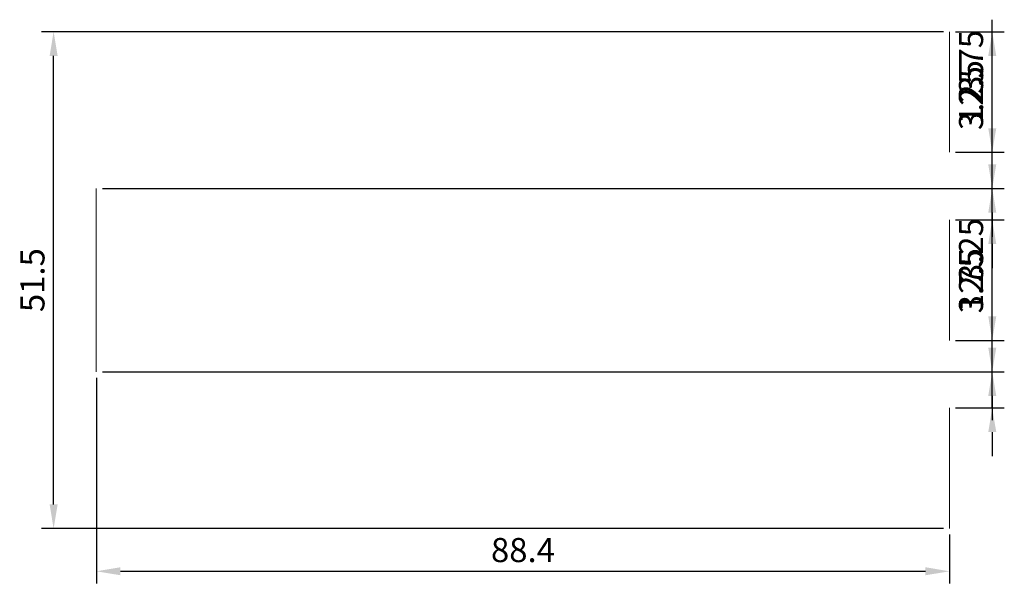
# Model space of a CAD drawing. Units: millimetres. Extents: x 330 to 432, y -31 to 27.
import ezdxf

# ---------------------------------------------------------------- set-up
doc = ezdxf.new("R2010")
doc.units = ezdxf.units.MM
doc.layers.add('M-CONS', color=8, linetype='Continuous', lineweight=13)
doc.layers.add('M-DIMS', color=2, linetype='Continuous', lineweight=18)
doc.dimstyles.new('ISO-25', dxfattribs={"dimtxt": 2.5, "dimasz": 2.5, "dimexe": 1.25, "dimexo": 0.625, "dimtad": 1, "dimtxsty": 'Standard', "dimcen": 2.5, "dimadec": 0, "dimazin": 0, "dimtfac": 1, "dimtmove": 0, "dimatfit": 3, "dimfxl": 1, "dimarcsym": 0})

# ---------------------------------------------------------------- blocks, each defined once
blk = doc.blocks.new('*D1')
at = {"layer": 'Defpoints', "color": 0, "transparency": 16777216}
for p in [(338.36, -9.5), (426.76, -25.75), (426.76, -30.18)]:
    blk.add_point(p, dxfattribs=at)
at = {"layer": 'M-DIMS', "color": 0, "lineweight": -2, "transparency": 16777216}
for p, q in [((338.36, -10.12), (338.36, -31.43)), ((426.76, -26.38), (426.76, -31.43)), ((340.86, -30.18), (424.26, -30.18))]:
    blk.add_line(p, q, dxfattribs=at)
at = {"layer": 'M-DIMS', "color": 0, "transparency": 16777216}
for points in [[(340.86, -29.76), (340.86, -30.59), (338.36, -30.18)], [(424.26, -29.76), (424.26, -30.59), (426.76, -30.18)]]:
    blk.add_solid(points, dxfattribs=at)
at = {"layer": 'M-DIMS', "color": 0, "transparency": 16777216, "insert": (382.56, -28.3), "char_height": 2.5, "attachment_point": 5}
blk.add_mtext('88.4', dxfattribs=at)
blk = doc.blocks.new('*D2')
at = {"layer": 'Defpoints', "color": 0, "transparency": 16777216}
for p in [(333.93, 25.75), (426.76, 25.75), (426.76, -25.75)]:
    blk.add_point(p, dxfattribs=at)
at = {"layer": 'M-DIMS', "color": 0, "lineweight": -2, "transparency": 16777216}
for p, q in [((426.13, 25.75), (332.68, 25.75)), ((333.93, -23.25), (333.93, 23.25)), ((426.13, -25.75), (332.68, -25.75))]:
    blk.add_line(p, q, dxfattribs=at)
at = {"layer": 'M-DIMS', "color": 0, "transparency": 16777216}
for points in [[(333.52, 23.25), (334.35, 23.25), (333.93, 25.75)], [(333.52, -23.25), (334.35, -23.25), (333.93, -25.75)]]:
    blk.add_solid(points, dxfattribs=at)
at = {"layer": 'M-DIMS', "color": 0, "transparency": 16777216, "insert": (332.06, 0), "char_height": 2.5, "attachment_point": 5, "rotation": 90}
blk.add_mtext('51.5', dxfattribs=at)
blk = doc.blocks.new('*D3')
at = {"layer": 'Defpoints', "color": 0, "transparency": 16777216}
for p in [(426.76, 25.75), (431.18, 25.75), (426.76, 13.25)]:
    blk.add_point(p, dxfattribs=at)
at = {"layer": 'M-DIMS', "color": 0, "lineweight": -2, "transparency": 16777216}
for p, q in [((427.38, 25.75), (432.43, 25.75)), ((431.18, 15.75), (431.18, 23.25)), ((427.38, 13.25), (432.43, 13.25))]:
    blk.add_line(p, q, dxfattribs=at)
at = {"layer": 'M-DIMS', "color": 0, "transparency": 16777216}
for points in [[(430.77, 23.25), (431.6, 23.25), (431.18, 25.75)], [(430.77, 15.75), (431.6, 15.75), (431.18, 13.25)]]:
    blk.add_solid(points, dxfattribs=at)
at = {"layer": 'M-DIMS', "color": 0, "transparency": 16777216, "insert": (429.31, 19.5), "char_height": 2.5, "attachment_point": 5, "rotation": 90}
blk.add_mtext('12.5', dxfattribs=at)
blk = doc.blocks.new('*D4')
at = {"layer": 'Defpoints', "color": 0, "transparency": 16777216}
for p in [(426.76, 13.25), (431.18, 13.25), (338.36, 9.5)]:
    blk.add_point(p, dxfattribs=at)
at = {"layer": 'M-DIMS', "color": 0, "lineweight": -2, "transparency": 16777216}
for p, q in [((431.18, 15.75), (431.18, 27)), ((427.38, 13.25), (432.43, 13.25)), ((431.18, 9.5), (431.18, 13.25)), ((338.98, 9.5), (432.43, 9.5)), ((431.18, 7), (431.18, 4.5))]:
    blk.add_line(p, q, dxfattribs=at)
at = {"layer": 'M-DIMS', "color": 0, "transparency": 16777216}
for points in [[(430.77, 15.75), (431.6, 15.75), (431.18, 13.25)], [(430.77, 7), (431.6, 7), (431.18, 9.5)]]:
    blk.add_solid(points, dxfattribs=at)
at = {"layer": 'M-DIMS', "color": 0, "transparency": 16777216, "insert": (429.31, 22.62), "char_height": 2.5, "attachment_point": 5, "rotation": 90}
blk.add_mtext('3.75', dxfattribs=at)
blk = doc.blocks.new('*D5')
at = {"layer": 'Defpoints', "color": 0, "transparency": 16777216}
for p in [(338.36, 9.5), (431.18, 9.5), (426.76, 6.25)]:
    blk.add_point(p, dxfattribs=at)
at = {"layer": 'M-DIMS', "color": 0, "lineweight": -2, "transparency": 16777216}
for p, q in [((431.18, 12), (431.18, 23.25)), ((338.98, 9.5), (432.43, 9.5)), ((431.18, 6.25), (431.18, 9.5)), ((427.38, 6.25), (432.43, 6.25)), ((431.18, 3.75), (431.18, 1.25))]:
    blk.add_line(p, q, dxfattribs=at)
at = {"layer": 'M-DIMS', "color": 0, "transparency": 16777216}
for points in [[(430.77, 12), (431.6, 12), (431.18, 9.5)], [(430.77, 3.75), (431.6, 3.75), (431.18, 6.25)]]:
    blk.add_solid(points, dxfattribs=at)
at = {"layer": 'M-DIMS', "color": 0, "transparency": 16777216, "insert": (429.31, 18.87), "char_height": 2.5, "attachment_point": 5, "rotation": 90}
blk.add_mtext('3.25', dxfattribs=at)
blk = doc.blocks.new('*D6')
at = {"layer": 'Defpoints', "color": 0, "transparency": 16777216}
for p in [(426.76, 6.25), (431.18, 6.25), (426.76, -6.25)]:
    blk.add_point(p, dxfattribs=at)
at = {"layer": 'M-DIMS', "color": 0, "lineweight": -2, "transparency": 16777216}
for p, q in [((427.38, 6.25), (432.43, 6.25)), ((431.18, -3.75), (431.18, 3.75)), ((427.38, -6.25), (432.43, -6.25))]:
    blk.add_line(p, q, dxfattribs=at)
at = {"layer": 'M-DIMS', "color": 0, "transparency": 16777216}
for points in [[(430.77, 3.75), (431.6, 3.75), (431.18, 6.25)], [(430.77, -3.75), (431.6, -3.75), (431.18, -6.25)]]:
    blk.add_solid(points, dxfattribs=at)
at = {"layer": 'M-DIMS', "color": 0, "transparency": 16777216, "insert": (429.31, 0), "char_height": 2.5, "attachment_point": 5, "rotation": 90}
blk.add_mtext('12.5', dxfattribs=at)
blk = doc.blocks.new('*D7')
at = {"layer": 'Defpoints', "color": 0, "transparency": 16777216}
for p in [(426.76, -6.25), (431.18, -6.25), (338.36, -9.5)]:
    blk.add_point(p, dxfattribs=at)
at = {"layer": 'M-DIMS', "color": 0, "lineweight": -2, "transparency": 16777216}
for p, q in [((431.18, -3.75), (431.18, 7.5)), ((427.38, -6.25), (432.43, -6.25)), ((431.18, -9.5), (431.18, -6.25)), ((338.98, -9.5), (432.43, -9.5)), ((431.18, -12), (431.18, -14.5))]:
    blk.add_line(p, q, dxfattribs=at)
at = {"layer": 'M-DIMS', "color": 0, "transparency": 16777216}
for points in [[(430.77, -3.75), (431.6, -3.75), (431.18, -6.25)], [(430.77, -12), (431.6, -12), (431.18, -9.5)]]:
    blk.add_solid(points, dxfattribs=at)
at = {"layer": 'M-DIMS', "color": 0, "transparency": 16777216, "insert": (429.31, 3.12), "char_height": 2.5, "attachment_point": 5, "rotation": 90}
blk.add_mtext('3.25', dxfattribs=at)
blk = doc.blocks.new('*D8')
at = {"layer": 'Defpoints', "color": 0, "transparency": 16777216}
for p in [(338.36, -9.5), (431.18, -9.5), (426.76, -13.25)]:
    blk.add_point(p, dxfattribs=at)
at = {"layer": 'M-DIMS', "color": 0, "lineweight": -2, "transparency": 16777216}
for p, q in [((431.18, -7), (431.18, 4.25)), ((338.98, -9.5), (432.43, -9.5)), ((431.18, -13.25), (431.18, -9.5)), ((427.38, -13.25), (432.43, -13.25)), ((431.18, -15.75), (431.18, -18.25))]:
    blk.add_line(p, q, dxfattribs=at)
at = {"layer": 'M-DIMS', "color": 0, "transparency": 16777216}
for points in [[(430.77, -7), (431.6, -7), (431.18, -9.5)], [(430.77, -15.75), (431.6, -15.75), (431.18, -13.25)]]:
    blk.add_solid(points, dxfattribs=at)
at = {"layer": 'M-DIMS', "color": 0, "transparency": 16777216, "insert": (429.31, -0.13), "char_height": 2.5, "attachment_point": 5, "rotation": 90}
blk.add_mtext('3.75', dxfattribs=at)

msp = doc.modelspace()

# ---------------------------------------------------------------- linework, layer by layer
at = {"layer": 'M-CONS', "extrusion": (1, 0, 0)}
for centre in [(19.5, 155.769, 426.757), (0, 136.269, 426.757), (0, 175.269, 426.757), (-19.5, 155.769, 426.757)]:
    msp.add_circle(centre, 6.25, dxfattribs=at)
at = {"layer": 'M-CONS', "extrusion": (-1, 0, 0)}
msp.add_circle((0, 155.769, -338.357), 9.5, dxfattribs=at)

# ---------------------------------------------------------------- dimensions: what is measured, and where the dimension line sits
at = {"layer": 'M-DIMS'}
for base, p1, p2, override, picture, middle in [((431.182, 13.25), (338.357, 9.5), (426.757, 13.25), {"dimdec": 2, "dimlfac": 1, "dimrnd": 0, "dimzin": 0, "dimdsep": 46, "dimlunit": 2}, '*D4', (429.307, 22.625)), ((333.932, 25.75), (426.757, -25.75), (426.757, 25.75), {"dimdec": 1, "dimlfac": 1, "dimrnd": 0, "dimzin": 0, "dimdsep": 46, "dimlunit": 2}, '*D2', (332.057, 0)), ((431.182, 25.75), (426.757, 13.25), (426.757, 25.75), {"dimdec": 1, "dimlfac": 1, "dimrnd": 0, "dimzin": 0, "dimdsep": 46, "dimlunit": 2}, '*D3', (429.307, 19.5)), ((431.182, 9.5), (426.757, 6.25), (338.357, 9.5), {"dimdec": 2, "dimlfac": 1, "dimrnd": 0, "dimzin": 0, "dimdsep": 46, "dimlunit": 2}, '*D5', (429.307, 18.875)), ((431.182, -6.25), (338.357, -9.5), (426.757, -6.25), {"dimdec": 2, "dimlfac": 1, "dimrnd": 0, "dimzin": 0, "dimdsep": 46, "dimlunit": 2}, '*D7', (429.307, 3.125)), ((431.182, 6.25), (426.757, -6.25), (426.757, 6.25), {"dimdec": 1, "dimlfac": 1, "dimrnd": 0, "dimzin": 0, "dimdsep": 46, "dimlunit": 2}, '*D6', (429.307, 0)), ((431.182, -9.5), (426.757, -13.25), (338.357, -9.5), {"dimdec": 2, "dimlfac": 1, "dimrnd": 0, "dimzin": 0, "dimdsep": 46, "dimlunit": 2}, '*D8', (429.307, -0.125))]:
    dim = msp.add_linear_dim(base=base, p1=p1, p2=p2, angle=90, dimstyle='ISO-25', override=override, dxfattribs=at)
    dim.commit()
    dim.dimension.update_dxf_attribs({"geometry": picture, "text_midpoint": middle})
dim = msp.add_linear_dim(base=(426.757, -30.175), p1=(338.357, -9.5), p2=(426.757, -25.75), dimstyle='ISO-25', override={"dimdec": 1, "dimlfac": 1, "dimrnd": 0, "dimzin": 0, "dimdsep": 46, "dimlunit": 2}, dxfattribs=at)
dim.commit()
dim.dimension.update_dxf_attribs({"geometry": '*D1', "text_midpoint": (382.557, -28.3)})

doc.saveas('drawing.dxf')
